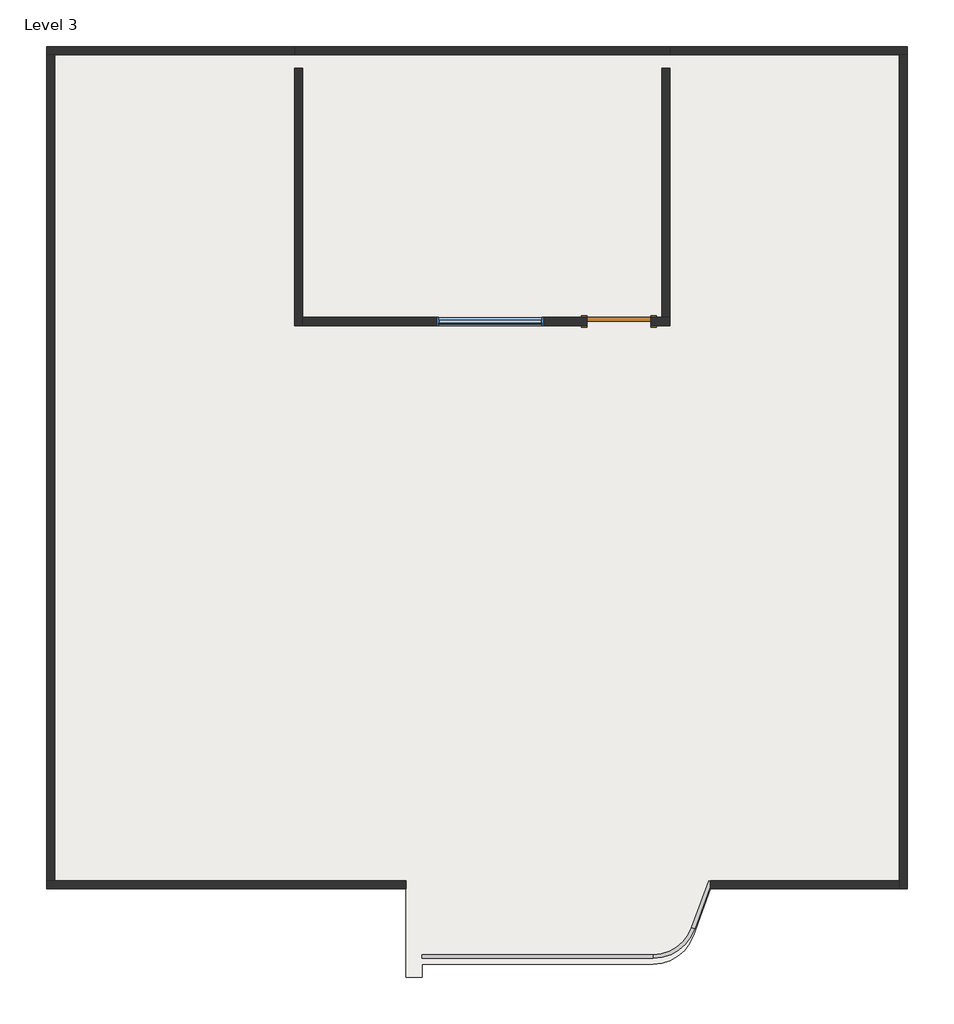
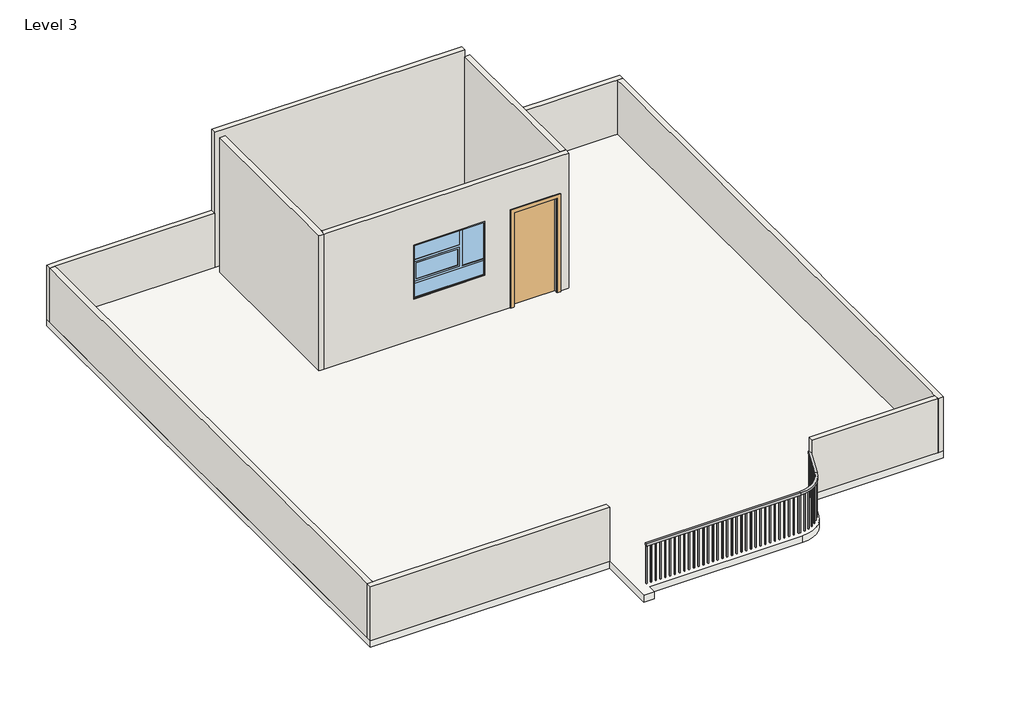
# One storey: 10 walls, 1 door, 1 railing, 1 slab, 1 window.
"""IFC4 building model written with IfcOpenShell, lengths in millimetres."""

from ifc_helpers import new_model, si_unit, point, frame, frame_2d, origin, place, context, project, spatial, polyline, circle_curve, trimmed, segment, composite_curve, outline, extrude, faceted_brep, transform, mapped, element, save
from ifc_brep_helpers import plane_surface, cylinder_surface, revolved_surface, advanced_brep
from components import door_e5f9f3c4, window_awning_variable_5_x4_55050b8f

model = new_model("IFC4")

# Units and contexts
model_context = context("Model", 3, world=origin())
ifc_project = project(units=[si_unit("LENGTHUNIT", "METRE", prefix="MILLI")], contexts=[model_context])

# Site, building, storey
site = spatial("IfcSite", under=ifc_project)
building = spatial("IfcBuilding", under=site)
storey = spatial("IfcBuildingStorey", under=building, Name="Level 3", Elevation=6400.8)

# Door
placement = place(None, origin())
door_shape = door_e5f9f3c4(model_context)
element("IfcDoor", 1, ObjectType="Single-Flush : 36\" x 84\"", at=placement, inside=storey, context=model_context, shape_type="MappedRepresentation", body=[
    mapped(door_shape, transform((-6761.6178125, 9626.366018, 6400.8), x_axis=(1.0, 0.0, 0.0), y_axis=(0.0, 1.0, 0.0), z_axis=(0.0, 0.0, 1.0))),
])

# Railing
element("IfcRailing", 2, ObjectType="Handrail - Rectangular", at=placement, inside=storey, context=model_context, shape_type="SolidModel", body=[
    advanced_brep(
    [(-9561.9678125, 634.766018, 7315.2), (-9561.9678125, 634.766018, 7264.4), (-9561.9678125, 583.966018, 7264.4), (-9561.9678125, 583.966018, 7315.2), (-6278.443289, 634.766018, 7315.2), (-6278.443289, 634.766018, 7264.4), (-6278.443289, 583.966018, 7264.4), (-6278.443289, 583.966018, 7315.2), (-5729.4748599, 1019.1578503, 7264.4), (-5729.4748599, 1019.1578503, 7315.2), (-5681.7384748, 1001.783227, 7264.4), (-5681.7384748, 1001.783227, 7315.2), (-5487.1815204, 1684.8533296, 7315.2), (-5439.4451352, 1667.4787064, 7315.2), (-5439.4451352, 1667.4787064, 7264.4), (-5487.1815204, 1684.8533296, 7264.4)],
    [
        (0, 1),
        (1, 2),
        (2, 3),
        (3, 0),
        (0, 4),
        (4, 5),
        (5, 1),
        (5, 6),
        (6, 2),
        (6, 7),
        (7, 3),
        (7, 4),
        (8, 5, circle_curve(frame((-6278.443289, 1218.966018, 7264.4), z_axis=(0.0, 0.0, -1.0), x_axis=(0.0, -1.0, 0.0)), 584.2)),
        (4, 9, circle_curve(frame((-6278.443289, 1218.966018, 7315.2), z_axis=(0.0, 0.0, 1.0), x_axis=(0.0, -1.0, 0.0)), 584.2)),
        (9, 8),
        (10, 6, circle_curve(frame((-6278.443289, 1218.966018, 7264.4), z_axis=(0.0, 0.0, -1.0), x_axis=(0.0, -1.0, 0.0)), 635.0)),
        (8, 10),
        (11, 7, circle_curve(frame((-6278.443289, 1218.966018, 7315.2), z_axis=(0.0, 0.0, -1.0), x_axis=(0.0, -1.0, 0.0)), 635.0)),
        (10, 11),
        (11, 9),
        (12, 13),
        (13, 14),
        (14, 15),
        (15, 12),
        (9, 12),
        (15, 8),
        (14, 10),
        (13, 11),
    ],
    [
        plane_surface(frame((-9561.9678125, 609.366018, 7315.2), z_axis=(-1.0, 0.0, 0.0), x_axis=(0.0, 1.0, 0.0))),
        plane_surface(frame((-9561.9678125, 634.766018, 7315.2), z_axis=(0.0, 1.0, 0.0), x_axis=(1.0, 0.0, 0.0))),
        plane_surface(frame((-9561.9678125, 634.766018, 7264.4), z_axis=(0.0, 0.0, -1.0), x_axis=(1.0, 0.0, 0.0))),
        plane_surface(frame((-9561.9678125, 583.966018, 7264.4), z_axis=(0.0, -1.0, 0.0), x_axis=(1.0, 0.0, 0.0))),
        plane_surface(frame((-9561.9678125, 583.966018, 7315.2), z_axis=(0.0, 0.0, 1.0), x_axis=(1.0, 0.0, 0.0))),
        revolved_surface(polyline([(-6278.443289, 634.766018, 7315.2), (-6278.443289, 634.766018, 7264.4)]), (-6278.443289, 1218.966018, 7315.2), (0.0, 0.0, 1.0)),
        plane_surface(frame((-6278.443289, 1218.966018, 7264.4), z_axis=(0.0, 0.0, -1.0), x_axis=(0.0, -1.0, 0.0))),
        cylinder_surface(frame((-6278.443289, 1218.966018, 7315.2), z_axis=(0.0, 0.0, 1.0), x_axis=(0.0, -1.0, 0.0)), 635.0),
        plane_surface(frame((-6278.443289, 1218.966018, 7315.2), z_axis=(0.0, 0.0, 1.0), x_axis=(0.0, -1.0, 0.0))),
        plane_surface(frame((-5463.3133278, 1676.166018, 7315.2), z_axis=(0.3420201433256705, 0.9396926207859078, 0.0), x_axis=(0.9396926207859078, -0.3420201433256705, 0.0))),
        plane_surface(frame((-5729.4748599, 1019.1578503, 7315.2), z_axis=(-0.9396926207859079, 0.3420201433256703, 0.0), x_axis=(0.3420201433256703, 0.9396926207859079, 0.0))),
        plane_surface(frame((-5729.4748599, 1019.1578503, 7264.4), z_axis=(0.0, 0.0, -1.0), x_axis=(0.3420201433256703, 0.9396926207859079, 0.0))),
        plane_surface(frame((-5681.7384748, 1001.783227, 7264.4), z_axis=(0.9396926207859079, -0.34202014332567027, 0.0), x_axis=(0.34202014332567027, 0.9396926207859079, 0.0))),
        plane_surface(frame((-5681.7384748, 1001.783227, 7315.2), z_axis=(0.0, 0.0, 1.0), x_axis=(0.34202014332567027, 0.9396926207859079, 0.0))),
    ],
    [
        (0, [[1, 2, 3, 4]]),
        (1, [[-1, 5, 6, 7]]),
        (2, [[-2, -7, 8, 9]]),
        (3, [[-3, -9, 10, 11]]),
        (4, [[-4, -11, 12, -5]]),
        (5, [[13, -6, 14, 15]]),
        (6, [[16, -8, -13, 17]]),
        (7, [[18, -10, -16, 19]]),
        (8, [[-14, -12, -18, 20]]),
        (9, [[21, 22, 23, 24]]),
        (10, [[-15, 25, -24, 26]]),
        (11, [[-17, -26, -23, 27]]),
        (12, [[-19, -27, -22, 28]]),
        (13, [[-20, -28, -21, -25]]),
    ],
),
    extrude(outline(polyline([(-5491.4183577, 1571.0988462), (-5509.3195021, 1577.6143299), (-5502.8040184, 1595.5154743), (-5484.9028739, 1588.9999906), (-5491.4183577, 1571.0988462)])), frame((0.0, 0.0, 6400.8), z_axis=(0.0, 0.0, 1.0), x_axis=(1.0, 0.0, 0.0)), (0.0, 0.0, 1.0), 863.6),
    extrude(outline(polyline([(-5526.1676042, 1475.6260759), (-5544.0687486, 1482.1415596), (-5537.5532649, 1500.0427041), (-5519.6521205, 1493.5272203), (-5526.1676042, 1475.6260759)])), frame((0.0, 0.0, 6400.8), z_axis=(0.0, 0.0, 1.0), x_axis=(1.0, 0.0, 0.0)), (0.0, 0.0, 1.0), 863.6),
    extrude(outline(polyline([(-5560.9168508, 1380.1533056), (-5578.8179952, 1386.6687894), (-5572.3025115, 1404.5699338), (-5554.4013671, 1398.0544501), (-5560.9168508, 1380.1533056)])), frame((0.0, 0.0, 6400.8), z_axis=(0.0, 0.0, 1.0), x_axis=(1.0, 0.0, 0.0)), (0.0, 0.0, 1.0), 863.6),
    extrude(outline(polyline([(-5595.6660973, 1284.6805354), (-5613.5672418, 1291.1960191), (-5607.051758, 1309.0971635), (-5589.1506136, 1302.5816798), (-5595.6660973, 1284.6805354)])), frame((0.0, 0.0, 6400.8), z_axis=(0.0, 0.0, 1.0), x_axis=(1.0, 0.0, 0.0)), (0.0, 0.0, 1.0), 863.6),
    extrude(outline(polyline([(-5630.4153439, 1189.2077651), (-5648.3164883, 1195.7232488), (-5641.8010046, 1213.6243932), (-5623.8998602, 1207.1089095), (-5630.4153439, 1189.2077651)])), frame((0.0, 0.0, 6400.8), z_axis=(0.0, 0.0, 1.0), x_axis=(1.0, 0.0, 0.0)), (0.0, 0.0, 1.0), 863.6),
    extrude(outline(polyline([(-5665.1645905, 1093.7349948), (-5683.0657349, 1100.2504785), (-5676.5502512, 1118.151623), (-5658.6491067, 1111.6361392), (-5665.1645905, 1093.7349948)])), frame((0.0, 0.0, 6400.8), z_axis=(0.0, 0.0, 1.0), x_axis=(1.0, 0.0, 0.0)), (0.0, 0.0, 1.0), 863.6),
    extrude(outline(polyline([(-5712.9373242, 966.7567894), (-5730.452751, 974.2476053), (-5722.9619352, 991.7630322), (-5705.4465083, 984.2722163), (-5712.9373242, 966.7567894)])), frame((0.0, 0.0, 6400.8), z_axis=(0.0, 0.0, 1.0), x_axis=(1.0, 0.0, 0.0)), (0.0, 0.0, 1.0), 863.6),
    extrude(outline(polyline([(-5762.613945, 876.4363417), (-5778.6439673, 886.7291007), (-5768.3512083, 902.7591229), (-5752.3211861, 892.466364), (-5762.613945, 876.4363417)])), frame((0.0, 0.0, 6400.8), z_axis=(0.0, 0.0, 1.0), x_axis=(1.0, 0.0, 0.0)), (0.0, 0.0, 1.0), 863.6),
    extrude(outline(polyline([(-5826.5860214, 795.6086028), (-5840.6863905, 808.4180561), (-5827.8769372, 822.5184252), (-5813.7765681, 809.7089719), (-5826.5860214, 795.6086028)])), frame((0.0, 0.0, 6400.8), z_axis=(0.0, 0.0, 1.0), x_axis=(1.0, 0.0, 0.0)), (0.0, 0.0, 1.0), 863.6),
    extrude(outline(polyline([(-5903.0806608, 726.5135953), (-5914.8606056, 741.4847476), (-5899.8894533, 753.2646924), (-5888.1095085, 738.29354), (-5903.0806608, 726.5135953)])), frame((0.0, 0.0, 6400.8), z_axis=(0.0, 0.0, 1.0), x_axis=(1.0, 0.0, 0.0)), (0.0, 0.0, 1.0), 863.6),
    extrude(outline(polyline([(-5989.9779263, 671.0661861), (-5999.1109828, 687.7841339), (-5982.393035, 696.9171904), (-5973.2599785, 680.1992426), (-5989.9779263, 671.0661861)])), frame((0.0, 0.0, 6400.8), z_axis=(0.0, 0.0, 1.0), x_axis=(1.0, 0.0, 0.0)), (0.0, 0.0, 1.0), 863.6),
    extrude(outline(polyline([(-6084.8695873, 630.8030191), (-6091.1026462, 648.8044489), (-6073.1012164, 655.0375079), (-6066.8681574, 637.0360781), (-6084.8695873, 630.8030191)])), frame((0.0, 0.0, 6400.8), z_axis=(0.0, 0.0, 1.0), x_axis=(1.0, 0.0, 0.0)), (0.0, 0.0, 1.0), 863.6),
    extrude(outline(polyline([(-6185.1258601, 606.8399291), (-6188.2861815, 625.6259576), (-6169.5001529, 628.786279), (-6166.3398316, 610.0002504), (-6185.1258601, 606.8399291)])), frame((0.0, 0.0, 6400.8), z_axis=(0.0, 0.0, 1.0), x_axis=(1.0, 0.0, 0.0)), (0.0, 0.0, 1.0), 863.6),
    extrude(outline(polyline([(-6320.2928125, 599.841018), (-6320.2928125, 618.891018), (-6301.2428125, 618.891018), (-6301.2428125, 599.841018), (-6320.2928125, 599.841018)])), frame((0.0, 0.0, 6400.8), z_axis=(0.0, 0.0, 1.0), x_axis=(1.0, 0.0, 0.0)), (0.0, 0.0, 1.0), 863.6),
    extrude(outline(polyline([(-6421.8928125, 599.841018), (-6421.8928125, 618.891018), (-6402.8428125, 618.891018), (-6402.8428125, 599.841018), (-6421.8928125, 599.841018)])), frame((0.0, 0.0, 6400.8), z_axis=(0.0, 0.0, 1.0), x_axis=(1.0, 0.0, 0.0)), (0.0, 0.0, 1.0), 863.6),
    extrude(outline(polyline([(-6523.4928125, 599.841018), (-6523.4928125, 618.891018), (-6504.4428125, 618.891018), (-6504.4428125, 599.841018), (-6523.4928125, 599.841018)])), frame((0.0, 0.0, 6400.8), z_axis=(0.0, 0.0, 1.0), x_axis=(1.0, 0.0, 0.0)), (0.0, 0.0, 1.0), 863.6),
    extrude(outline(polyline([(-6625.0928125, 599.841018), (-6625.0928125, 618.891018), (-6606.0428125, 618.891018), (-6606.0428125, 599.841018), (-6625.0928125, 599.841018)])), frame((0.0, 0.0, 6400.8), z_axis=(0.0, 0.0, 1.0), x_axis=(1.0, 0.0, 0.0)), (0.0, 0.0, 1.0), 863.6),
    extrude(outline(polyline([(-6726.6928125, 599.841018), (-6726.6928125, 618.891018), (-6707.6428125, 618.891018), (-6707.6428125, 599.841018), (-6726.6928125, 599.841018)])), frame((0.0, 0.0, 6400.8), z_axis=(0.0, 0.0, 1.0), x_axis=(1.0, 0.0, 0.0)), (0.0, 0.0, 1.0), 863.6),
    extrude(outline(polyline([(-6828.2928125, 599.841018), (-6828.2928125, 618.891018), (-6809.2428125, 618.891018), (-6809.2428125, 599.841018), (-6828.2928125, 599.841018)])), frame((0.0, 0.0, 6400.8), z_axis=(0.0, 0.0, 1.0), x_axis=(1.0, 0.0, 0.0)), (0.0, 0.0, 1.0), 863.6),
    extrude(outline(polyline([(-6929.8928125, 599.841018), (-6929.8928125, 618.891018), (-6910.8428125, 618.891018), (-6910.8428125, 599.841018), (-6929.8928125, 599.841018)])), frame((0.0, 0.0, 6400.8), z_axis=(0.0, 0.0, 1.0), x_axis=(1.0, 0.0, 0.0)), (0.0, 0.0, 1.0), 863.6),
    extrude(outline(polyline([(-7031.4928125, 599.841018), (-7031.4928125, 618.891018), (-7012.4428125, 618.891018), (-7012.4428125, 599.841018), (-7031.4928125, 599.841018)])), frame((0.0, 0.0, 6400.8), z_axis=(0.0, 0.0, 1.0), x_axis=(1.0, 0.0, 0.0)), (0.0, 0.0, 1.0), 863.6),
    extrude(outline(polyline([(-7133.0928125, 599.841018), (-7133.0928125, 618.891018), (-7114.0428125, 618.891018), (-7114.0428125, 599.841018), (-7133.0928125, 599.841018)])), frame((0.0, 0.0, 6400.8), z_axis=(0.0, 0.0, 1.0), x_axis=(1.0, 0.0, 0.0)), (0.0, 0.0, 1.0), 863.6),
    extrude(outline(polyline([(-7234.6928125, 599.841018), (-7234.6928125, 618.891018), (-7215.6428125, 618.891018), (-7215.6428125, 599.841018), (-7234.6928125, 599.841018)])), frame((0.0, 0.0, 6400.8), z_axis=(0.0, 0.0, 1.0), x_axis=(1.0, 0.0, 0.0)), (0.0, 0.0, 1.0), 863.6),
    extrude(outline(polyline([(-7336.2928125, 599.841018), (-7336.2928125, 618.891018), (-7317.2428125, 618.891018), (-7317.2428125, 599.841018), (-7336.2928125, 599.841018)])), frame((0.0, 0.0, 6400.8), z_axis=(0.0, 0.0, 1.0), x_axis=(1.0, 0.0, 0.0)), (0.0, 0.0, 1.0), 863.6),
    extrude(outline(polyline([(-7437.8928125, 599.841018), (-7437.8928125, 618.891018), (-7418.8428125, 618.891018), (-7418.8428125, 599.841018), (-7437.8928125, 599.841018)])), frame((0.0, 0.0, 6400.8), z_axis=(0.0, 0.0, 1.0), x_axis=(1.0, 0.0, 0.0)), (0.0, 0.0, 1.0), 863.6),
    extrude(outline(polyline([(-7539.4928125, 599.841018), (-7539.4928125, 618.891018), (-7520.4428125, 618.891018), (-7520.4428125, 599.841018), (-7539.4928125, 599.841018)])), frame((0.0, 0.0, 6400.8), z_axis=(0.0, 0.0, 1.0), x_axis=(1.0, 0.0, 0.0)), (0.0, 0.0, 1.0), 863.6),
    extrude(outline(polyline([(-7641.0928125, 599.841018), (-7641.0928125, 618.891018), (-7622.0428125, 618.891018), (-7622.0428125, 599.841018), (-7641.0928125, 599.841018)])), frame((0.0, 0.0, 6400.8), z_axis=(0.0, 0.0, 1.0), x_axis=(1.0, 0.0, 0.0)), (0.0, 0.0, 1.0), 863.6),
    extrude(outline(polyline([(-7742.6928125, 599.841018), (-7742.6928125, 618.891018), (-7723.6428125, 618.891018), (-7723.6428125, 599.841018), (-7742.6928125, 599.841018)])), frame((0.0, 0.0, 6400.8), z_axis=(0.0, 0.0, 1.0), x_axis=(1.0, 0.0, 0.0)), (0.0, 0.0, 1.0), 863.6),
    extrude(outline(polyline([(-7844.2928125, 599.841018), (-7844.2928125, 618.891018), (-7825.2428125, 618.891018), (-7825.2428125, 599.841018), (-7844.2928125, 599.841018)])), frame((0.0, 0.0, 6400.8), z_axis=(0.0, 0.0, 1.0), x_axis=(1.0, 0.0, 0.0)), (0.0, 0.0, 1.0), 863.6),
    extrude(outline(polyline([(-7945.8928125, 599.841018), (-7945.8928125, 618.891018), (-7926.8428125, 618.891018), (-7926.8428125, 599.841018), (-7945.8928125, 599.841018)])), frame((0.0, 0.0, 6400.8), z_axis=(0.0, 0.0, 1.0), x_axis=(1.0, 0.0, 0.0)), (0.0, 0.0, 1.0), 863.6),
    extrude(outline(polyline([(-8047.4928125, 599.841018), (-8047.4928125, 618.891018), (-8028.4428125, 618.891018), (-8028.4428125, 599.841018), (-8047.4928125, 599.841018)])), frame((0.0, 0.0, 6400.8), z_axis=(0.0, 0.0, 1.0), x_axis=(1.0, 0.0, 0.0)), (0.0, 0.0, 1.0), 863.6),
    extrude(outline(polyline([(-8149.0928125, 599.841018), (-8149.0928125, 618.891018), (-8130.0428125, 618.891018), (-8130.0428125, 599.841018), (-8149.0928125, 599.841018)])), frame((0.0, 0.0, 6400.8), z_axis=(0.0, 0.0, 1.0), x_axis=(1.0, 0.0, 0.0)), (0.0, 0.0, 1.0), 863.6),
    extrude(outline(polyline([(-8250.6928125, 599.841018), (-8250.6928125, 618.891018), (-8231.6428125, 618.891018), (-8231.6428125, 599.841018), (-8250.6928125, 599.841018)])), frame((0.0, 0.0, 6400.8), z_axis=(0.0, 0.0, 1.0), x_axis=(1.0, 0.0, 0.0)), (0.0, 0.0, 1.0), 863.6),
    extrude(outline(polyline([(-8352.2928125, 599.841018), (-8352.2928125, 618.891018), (-8333.2428125, 618.891018), (-8333.2428125, 599.841018), (-8352.2928125, 599.841018)])), frame((0.0, 0.0, 6400.8), z_axis=(0.0, 0.0, 1.0), x_axis=(1.0, 0.0, 0.0)), (0.0, 0.0, 1.0), 863.6),
    extrude(outline(polyline([(-8453.8928125, 599.841018), (-8453.8928125, 618.891018), (-8434.8428125, 618.891018), (-8434.8428125, 599.841018), (-8453.8928125, 599.841018)])), frame((0.0, 0.0, 6400.8), z_axis=(0.0, 0.0, 1.0), x_axis=(1.0, 0.0, 0.0)), (0.0, 0.0, 1.0), 863.6),
    extrude(outline(polyline([(-8555.4928125, 599.841018), (-8555.4928125, 618.891018), (-8536.4428125, 618.891018), (-8536.4428125, 599.841018), (-8555.4928125, 599.841018)])), frame((0.0, 0.0, 6400.8), z_axis=(0.0, 0.0, 1.0), x_axis=(1.0, 0.0, 0.0)), (0.0, 0.0, 1.0), 863.6),
    extrude(outline(polyline([(-8657.0928125, 599.841018), (-8657.0928125, 618.891018), (-8638.0428125, 618.891018), (-8638.0428125, 599.841018), (-8657.0928125, 599.841018)])), frame((0.0, 0.0, 6400.8), z_axis=(0.0, 0.0, 1.0), x_axis=(1.0, 0.0, 0.0)), (0.0, 0.0, 1.0), 863.6),
    extrude(outline(polyline([(-8758.6928125, 599.841018), (-8758.6928125, 618.891018), (-8739.6428125, 618.891018), (-8739.6428125, 599.841018), (-8758.6928125, 599.841018)])), frame((0.0, 0.0, 6400.8), z_axis=(0.0, 0.0, 1.0), x_axis=(1.0, 0.0, 0.0)), (0.0, 0.0, 1.0), 863.6),
    extrude(outline(polyline([(-8860.2928125, 599.841018), (-8860.2928125, 618.891018), (-8841.2428125, 618.891018), (-8841.2428125, 599.841018), (-8860.2928125, 599.841018)])), frame((0.0, 0.0, 6400.8), z_axis=(0.0, 0.0, 1.0), x_axis=(1.0, 0.0, 0.0)), (0.0, 0.0, 1.0), 863.6),
    extrude(outline(polyline([(-8961.8928125, 599.841018), (-8961.8928125, 618.891018), (-8942.8428125, 618.891018), (-8942.8428125, 599.841018), (-8961.8928125, 599.841018)])), frame((0.0, 0.0, 6400.8), z_axis=(0.0, 0.0, 1.0), x_axis=(1.0, 0.0, 0.0)), (0.0, 0.0, 1.0), 863.6),
    extrude(outline(polyline([(-9063.4928125, 599.841018), (-9063.4928125, 618.891018), (-9044.4428125, 618.891018), (-9044.4428125, 599.841018), (-9063.4928125, 599.841018)])), frame((0.0, 0.0, 6400.8), z_axis=(0.0, 0.0, 1.0), x_axis=(1.0, 0.0, 0.0)), (0.0, 0.0, 1.0), 863.6),
    extrude(outline(polyline([(-9165.0928125, 599.841018), (-9165.0928125, 618.891018), (-9146.0428125, 618.891018), (-9146.0428125, 599.841018), (-9165.0928125, 599.841018)])), frame((0.0, 0.0, 6400.8), z_axis=(0.0, 0.0, 1.0), x_axis=(1.0, 0.0, 0.0)), (0.0, 0.0, 1.0), 863.6),
    extrude(outline(polyline([(-9266.6928125, 599.841018), (-9266.6928125, 618.891018), (-9247.6428125, 618.891018), (-9247.6428125, 599.841018), (-9266.6928125, 599.841018)])), frame((0.0, 0.0, 6400.8), z_axis=(0.0, 0.0, 1.0), x_axis=(1.0, 0.0, 0.0)), (0.0, 0.0, 1.0), 863.6),
    extrude(outline(polyline([(-9368.2928125, 599.841018), (-9368.2928125, 618.891018), (-9349.2428125, 618.891018), (-9349.2428125, 599.841018), (-9368.2928125, 599.841018)])), frame((0.0, 0.0, 6400.8), z_axis=(0.0, 0.0, 1.0), x_axis=(1.0, 0.0, 0.0)), (0.0, 0.0, 1.0), 863.6),
    extrude(outline(polyline([(-9469.8928125, 599.841018), (-9469.8928125, 618.891018), (-9450.8428125, 618.891018), (-9450.8428125, 599.841018), (-9469.8928125, 599.841018)])), frame((0.0, 0.0, 6400.8), z_axis=(0.0, 0.0, 1.0), x_axis=(1.0, 0.0, 0.0)), (0.0, 0.0, 1.0), 863.6),
    extrude(outline(polyline([(-5699.913837, 998.2622245), (-5717.8149815, 1004.7777083), (-5711.2994977, 1022.6788527), (-5693.3983533, 1016.163369), (-5699.913837, 998.2622245)])), frame((0.0, 0.0, 6400.8), z_axis=(0.0, 0.0, 1.0), x_axis=(1.0, 0.0, 0.0)), (0.0, 0.0, 1.0), 863.6),
    extrude(outline(polyline([(-6287.968289, 599.841018), (-6287.968289, 618.891018), (-6268.918289, 618.891018), (-6268.918289, 599.841018), (-6287.968289, 599.841018)])), frame((0.0, 0.0, 6400.8), z_axis=(0.0, 0.0, 1.0), x_axis=(1.0, 0.0, 0.0)), (0.0, 0.0, 1.0), 863.6),
    extrude(outline(polyline([(-5460.8782393, 1655.0071317), (-5478.7793837, 1661.5226154), (-5472.2639, 1679.4237599), (-5454.3627556, 1672.9082761), (-5460.8782393, 1655.0071317)])), frame((0.0, 0.0, 6400.8), z_axis=(0.0, 0.0, 1.0), x_axis=(1.0, 0.0, 0.0)), (0.0, 0.0, 1.0), 863.6),
    extrude(outline(polyline([(-9561.9678125, 599.841018), (-9561.9678125, 618.891018), (-9542.9178125, 618.891018), (-9542.9178125, 599.841018), (-9561.9678125, 599.841018)])), frame((0.0, 0.0, 6400.8), z_axis=(0.0, 0.0, 1.0), x_axis=(1.0, 0.0, 0.0)), (0.0, 0.0, 1.0), 863.6),
])

# Slab
element("IfcSlab", 3, ObjectType="6\" floor", at=placement, inside=storey, context=model_context, shape_type="SweptSolid", body=[
    extrude(outline(composite_curve([segment(polyline([(-2665.8678125, 13531.616018), (-2665.8678125, 1568.216018), (-5463.3133278, 1568.216018), (-5705.6066674, 902.5205386)]), True, "CONTINUOUS"), segment(trimmed(circle_curve(frame_2d((-6278.443289, 1111.016018)), 609.6), [point((-5705.6066674, 902.5205386))], [point((-6278.443289, 501.416018))], False, "CARTESIAN"), True, "CONTINUOUS"), segment(polyline([(-6278.443289, 501.416018), (-9561.9678125, 501.416018), (-9561.9678125, 310.916018), (-9790.5678125, 310.916018), (-9790.5678125, 1568.216018), (-14895.9678125, 1568.216018), (-14895.9678125, 13531.616018), (-2665.8678125, 13531.616018)]), True, "CONTINUOUS")], self_intersect=False)), frame((0.0, 0.0, 6248.4), z_axis=(0.0, 0.0, 1.0), x_axis=(1.0, 0.0, 0.0)), (0.0, 0.0, 1.0), 152.4),
])

# Walls
element("IfcWall", 4, ObjectType="4.5\" wall", at=placement, inside=storey, context=model_context, shape_type="Brep", body=[
    faceted_brep([(-2665.8678125, 13531.616018, 6400.8), (-6037.7178125, 13531.616018, 6400.8), (-6037.7178125, 13531.616018, 7620.0), (-2894.4678125, 13531.616018, 7620.0), (-2665.8678125, 13531.616018, 7620.0), (-2665.8678125, 13417.316018, 6400.8), (-2665.8678125, 13417.316018, 7620.0), (-2780.1678125, 13417.316018, 7620.0), (-2894.4678125, 13417.316018, 7620.0), (-6037.7178125, 13417.316018, 7620.0), (-6037.7178125, 13417.316018, 6400.8), (-2894.4678125, 13417.316018, 6400.8), (-2780.1678125, 13417.316018, 6400.8)], [[[0, 1, 2, 3, 4]], [[5, 6, 7, 8, 9, 10, 11, 12]], [[1, 0, 5, 12, 11, 10]], [[2, 1, 10, 9]], [[4, 3, 2, 9, 8, 7, 6]], [[0, 4, 6, 5]]]),
])
element("IfcWall", 5, ObjectType="4.5\" wall", at=placement, inside=storey, context=model_context, shape_type="Brep", body=[
    faceted_brep([(-2665.8678125, 1568.216018, 6400.8), (-2665.8678125, 1873.016018, 6400.8), (-2665.8678125, 5930.666018, 6400.8), (-2665.8678125, 6235.466018, 6400.8), (-2665.8678125, 9397.766018, 6400.8), (-2665.8678125, 9702.566018, 6400.8), (-2665.8678125, 13226.816018, 6400.8), (-2665.8678125, 13303.016018, 6400.8), (-2665.8678125, 13417.316018, 6400.8), (-2665.8678125, 13417.316018, 7620.0), (-2665.8678125, 13226.816018, 7620.0), (-2665.8678125, 9702.566018, 7620.0), (-2665.8678125, 9397.766018, 7620.0), (-2665.8678125, 6235.466018, 7620.0), (-2665.8678125, 5930.666018, 7620.0), (-2665.8678125, 1873.016018, 7620.0), (-2665.8678125, 1568.216018, 7620.0), (-2780.1678125, 1568.216018, 6400.8), (-2780.1678125, 1568.216018, 7620.0), (-2780.1678125, 1682.516018, 7620.0), (-2780.1678125, 1873.016018, 7620.0), (-2780.1678125, 5930.666018, 7620.0), (-2780.1678125, 6235.466018, 7620.0), (-2780.1678125, 9397.766018, 7620.0), (-2780.1678125, 9702.566018, 7620.0), (-2780.1678125, 13226.816018, 7620.0), (-2780.1678125, 13417.316018, 7620.0), (-2780.1678125, 13417.316018, 6400.8), (-2780.1678125, 13303.016018, 6400.8), (-2780.1678125, 13226.816018, 6400.8), (-2780.1678125, 9702.566018, 6400.8), (-2780.1678125, 9397.766018, 6400.8), (-2780.1678125, 6235.466018, 6400.8), (-2780.1678125, 5930.666018, 6400.8), (-2780.1678125, 1873.016018, 6400.8), (-2780.1678125, 1682.516018, 6400.8)], [[[0, 1, 2, 3, 4, 5, 6, 7, 8, 9, 10, 11, 12, 13, 14, 15, 16]], [[17, 18, 19, 20, 21, 22, 23, 24, 25, 26, 27, 28, 29, 30, 31, 32, 33, 34, 35]], [[8, 7, 6, 5, 4, 3, 2, 1, 0, 17, 35, 34, 33, 32, 31, 30, 29, 28, 27]], [[16, 15, 14, 13, 12, 11, 10, 9, 26, 25, 24, 23, 22, 21, 20, 19, 18]], [[9, 8, 27, 26]], [[0, 16, 18, 17]]]),
])
element("IfcWall", 6, ObjectType="4.5\" wall", at=placement, inside=storey, context=model_context, shape_type="Brep", body=[
    faceted_brep([(-5463.3133278, 1568.216018, 6400.8), (-2894.4678125, 1568.216018, 6400.8), (-2780.1678125, 1568.216018, 6400.8), (-2780.1678125, 1568.216018, 7620.0), (-2894.4678125, 1568.216018, 7620.0), (-5463.3133278, 1568.216018, 7620.0), (-5463.3133278, 1682.516018, 6400.8), (-5463.3133278, 1682.516018, 7620.0), (-2894.4678125, 1682.516018, 7620.0), (-2780.1678125, 1682.516018, 7620.0), (-2780.1678125, 1682.516018, 6400.8), (-2894.4678125, 1682.516018, 6400.8)], [[[0, 1, 2, 3, 4, 5]], [[6, 7, 8, 9, 10, 11]], [[2, 1, 0, 6, 11, 10]], [[5, 4, 3, 9, 8, 7]], [[0, 5, 7, 6]], [[3, 2, 10, 9]]]),
])
element("IfcWall", 7, ObjectType="4.5\" wall", at=placement, inside=storey, context=model_context, shape_type="Brep", body=[
    faceted_brep([(-14895.9678125, 1568.216018, 6400.8), (-14667.3678125, 1568.216018, 6400.8), (-9790.5678125, 1568.216018, 6400.8), (-9790.5678125, 1568.216018, 7218.0977729), (-9790.5678125, 1568.216018, 7620.0), (-14629.2678125, 1568.216018, 7620.0), (-14895.9678125, 1568.216018, 7620.0), (-14895.9678125, 1682.516018, 6400.8), (-14895.9678125, 1682.516018, 7620.0), (-14781.6678125, 1682.516018, 7620.0), (-14629.2678125, 1682.516018, 7620.0), (-9790.5678125, 1682.516018, 7620.0), (-9790.5678125, 1682.516018, 7218.0977729), (-9790.5678125, 1682.516018, 6400.8), (-14629.2678125, 1682.516018, 6400.8), (-14667.3678125, 1682.516018, 6400.8), (-14781.6678125, 1682.516018, 6400.8)], [[[0, 1, 2, 3, 4, 5, 6]], [[7, 8, 9, 10, 11, 12, 13, 14, 15, 16]], [[2, 1, 0, 7, 16, 15, 14, 13]], [[6, 5, 4, 11, 10, 9, 8]], [[0, 6, 8, 7]], [[4, 3, 2, 13, 12, 11]]]),
])
element("IfcWall", 8, ObjectType="4.5\" wall", at=placement, inside=storey, context=model_context, shape_type="Brep", body=[
    faceted_brep([(-14895.9678125, 13417.316018, 6400.8), (-14895.9678125, 9645.416018, 6400.8), (-14895.9678125, 9340.616018, 6400.8), (-14895.9678125, 6235.466018, 6400.8), (-14895.9678125, 5930.666018, 6400.8), (-14895.9678125, 1682.516018, 6400.8), (-14895.9678125, 1682.516018, 7620.0), (-14895.9678125, 1796.816018, 7620.0), (-14895.9678125, 5930.666018, 7620.0), (-14895.9678125, 6235.466018, 7620.0), (-14895.9678125, 9340.616018, 7620.0), (-14895.9678125, 9645.416018, 7620.0), (-14895.9678125, 13303.016018, 7620.0), (-14895.9678125, 13417.316018, 7620.0), (-14781.6678125, 13417.316018, 6400.8), (-14781.6678125, 13417.316018, 7620.0), (-14781.6678125, 13303.016018, 7620.0), (-14781.6678125, 9645.416018, 7620.0), (-14781.6678125, 9340.616018, 7620.0), (-14781.6678125, 6235.466018, 7620.0), (-14781.6678125, 5930.666018, 7620.0), (-14781.6678125, 1796.816018, 7620.0), (-14781.6678125, 1682.516018, 7620.0), (-14781.6678125, 1682.516018, 6400.8), (-14781.6678125, 1796.816018, 6400.8), (-14781.6678125, 5930.666018, 6400.8), (-14781.6678125, 6235.466018, 6400.8), (-14781.6678125, 9340.616018, 6400.8), (-14781.6678125, 9645.416018, 6400.8), (-14781.6678125, 13303.016018, 6400.8)], [[[0, 1, 2, 3, 4, 5, 6, 7, 8, 9, 10, 11, 12, 13]], [[14, 15, 16, 17, 18, 19, 20, 21, 22, 23, 24, 25, 26, 27, 28, 29]], [[5, 4, 3, 2, 1, 0, 14, 29, 28, 27, 26, 25, 24, 23]], [[13, 12, 11, 10, 9, 8, 7, 6, 22, 21, 20, 19, 18, 17, 16, 15]], [[6, 5, 23, 22]], [[0, 13, 15, 14]]]),
])
element("IfcWall", 9, ObjectType="4.5\" wall", at=placement, inside=storey, context=model_context, shape_type="Brep", body=[
    faceted_brep([(-11371.7178125, 13226.816018, 6400.8), (-11371.7178125, 9702.566018, 6400.8), (-11371.7178125, 9645.416018, 6400.8), (-11371.7178125, 9569.216018, 6400.8), (-11371.7178125, 9569.216018, 9448.8), (-11371.7178125, 9702.566018, 9448.8), (-11371.7178125, 13226.816018, 9448.8), (-11257.4178125, 13226.816018, 6400.8), (-11257.4178125, 13226.816018, 9448.8), (-11257.4178125, 9702.566018, 9448.8), (-11257.4178125, 9683.516018, 9448.8), (-11257.4178125, 9569.216018, 9448.8), (-11257.4178125, 9569.216018, 6400.8), (-11257.4178125, 9683.516018, 6400.8), (-11257.4178125, 9702.566018, 6400.8), (-11314.5678125, 13226.816018, 6400.8), (-11314.5678125, 9569.216018, 6400.8)], [[[0, 1, 2, 3, 4, 5, 6]], [[7, 8, 9, 10, 11, 12, 13, 14]], [[3, 2, 1, 0, 15, 7, 14, 13, 12, 16]], [[6, 5, 4, 11, 10, 9, 8]], [[0, 6, 8, 7, 15]], [[4, 3, 16, 12, 11]]]),
])
element("IfcWall", 10, ObjectType="4.5\" wall", at=placement, inside=storey, context=model_context, shape_type="Brep", body=[
    faceted_brep([(-6304.4178125, 9569.216018, 8534.4), (-6304.4178125, 9569.216018, 6400.8), (-6209.1678125, 9569.216018, 6400.8), (-6094.8678125, 9569.216018, 6400.8), (-6037.7178125, 9569.216018, 6400.8), (-6037.7178125, 9569.216018, 9448.8), (-6209.1678125, 9569.216018, 9448.8), (-11200.2678125, 9569.216018, 9448.8), (-11257.4178125, 9569.216018, 9448.8), (-11257.4178125, 9569.216018, 6400.8), (-11200.2678125, 9569.216018, 6400.8), (-7218.8178125, 9569.216018, 6400.8), (-7218.8178125, 9569.216018, 8534.4), (-9352.4178125, 9569.216018, 8534.4), (-7828.4178125, 9569.216018, 8534.4), (-7828.4178125, 9569.216018, 7315.2), (-9352.4178125, 9569.216018, 7315.2), (-6037.7178125, 9683.516018, 6400.8), (-6152.0178125, 9683.516018, 6400.8), (-6209.1678125, 9683.516018, 6400.8), (-6304.4178125, 9683.516018, 6400.8), (-6304.4178125, 9683.516018, 8534.4), (-7218.8178125, 9683.516018, 8534.4), (-7218.8178125, 9683.516018, 6400.8), (-11200.2678125, 9683.516018, 6400.8), (-11257.4178125, 9683.516018, 6400.8), (-11257.4178125, 9683.516018, 9448.8), (-11200.2678125, 9683.516018, 9448.8), (-6209.1678125, 9683.516018, 9448.8), (-6152.0178125, 9683.516018, 9448.8), (-6037.7178125, 9683.516018, 9448.8), (-9352.4178125, 9683.516018, 8534.4), (-9352.4178125, 9683.516018, 7315.2), (-7828.4178125, 9683.516018, 7315.2), (-7828.4178125, 9683.516018, 8534.4), (-6037.7178125, 9645.416018, 6400.8)], [[[0, 1, 2, 3, 4, 5, 6, 7, 8, 9, 10, 11, 12], [13, 14, 15, 16]], [[17, 18, 19, 20, 21, 22, 23, 24, 25, 26, 27, 28, 29, 30], [31, 32, 33, 34]], [[11, 10, 9, 25, 24, 23]], [[4, 3, 2, 1, 20, 19, 18, 17, 35]], [[8, 7, 6, 5, 30, 29, 28, 27, 26]], [[9, 8, 26, 25]], [[5, 4, 35, 17, 30]], [[21, 20, 1, 0]], [[22, 21, 0, 12]], [[23, 22, 12, 11]], [[32, 31, 13, 16]], [[33, 32, 16, 15]], [[34, 33, 15, 14]], [[31, 34, 14, 13]]]),
])
element("IfcWall", 11, ObjectType="4.5\" wall", at=placement, inside=storey, context=model_context, shape_type="Brep", body=[
    faceted_brep([(-6037.7178125, 9683.516018, 6400.8), (-6037.7178125, 9702.566018, 6400.8), (-6037.7178125, 13226.816018, 6400.8), (-6037.7178125, 13226.816018, 9448.8), (-6037.7178125, 9702.566018, 9448.8), (-6037.7178125, 9683.516018, 9448.8), (-6152.0178125, 9683.516018, 6400.8), (-6152.0178125, 9683.516018, 9448.8), (-6152.0178125, 9702.566018, 9448.8), (-6152.0178125, 13226.816018, 9448.8), (-6152.0178125, 13226.816018, 6400.8), (-6152.0178125, 9702.566018, 6400.8), (-6094.8678125, 13226.816018, 6400.8)], [[[0, 1, 2, 3, 4, 5]], [[6, 7, 8, 9, 10, 11]], [[2, 1, 0, 6, 11, 10, 12]], [[3, 2, 12, 10, 9]], [[5, 4, 3, 9, 8, 7]], [[0, 5, 7, 6]]]),
])
element("IfcWall", 12, ObjectType="4.5\" wall", at=placement, inside=storey, context=model_context, shape_type="Brep", body=[
    faceted_brep([(-11371.7178125, 13531.616018, 6400.8), (-14591.1678125, 13531.616018, 6400.8), (-14667.3678125, 13531.616018, 6400.8), (-14895.9678125, 13531.616018, 6400.8), (-14895.9678125, 13531.616018, 7620.0), (-14591.1678125, 13531.616018, 7620.0), (-11371.7178125, 13531.616018, 7620.0), (-11371.7178125, 13417.316018, 6400.8), (-11371.7178125, 13417.316018, 7620.0), (-14591.1678125, 13417.316018, 7620.0), (-14781.6678125, 13417.316018, 7620.0), (-14895.9678125, 13417.316018, 7620.0), (-14895.9678125, 13417.316018, 6400.8), (-14781.6678125, 13417.316018, 6400.8), (-14667.3678125, 13417.316018, 6400.8), (-14591.1678125, 13417.316018, 6400.8)], [[[0, 1, 2, 3, 4, 5, 6]], [[7, 8, 9, 10, 11, 12, 13, 14, 15]], [[3, 2, 1, 0, 7, 15, 14, 13, 12]], [[6, 5, 4, 11, 10, 9, 8]], [[0, 6, 8, 7]], [[4, 3, 12, 11]]]),
])
element("IfcWall", 13, ObjectType="4.5\" wall", at=placement, inside=storey, context=model_context, shape_type="Brep", body=[
    faceted_brep([(-6037.7178125, 13531.616018, 6400.8), (-11371.7178125, 13531.616018, 6400.8), (-11371.7178125, 13531.616018, 7620.0), (-11371.7178125, 13531.616018, 9448.8), (-6037.7178125, 13531.616018, 9448.8), (-6037.7178125, 13531.616018, 7620.0), (-6037.7178125, 13417.316018, 6400.8), (-6037.7178125, 13417.316018, 7620.0), (-6037.7178125, 13417.316018, 9448.8), (-6266.3178125, 13417.316018, 9448.8), (-9504.8178125, 13417.316018, 9448.8), (-9733.4178125, 13417.316018, 9448.8), (-11143.1178125, 13417.316018, 9448.8), (-11371.7178125, 13417.316018, 9448.8), (-11371.7178125, 13417.316018, 7620.0), (-11371.7178125, 13417.316018, 6400.8), (-11143.1178125, 13417.316018, 6400.8), (-9733.4178125, 13417.316018, 6400.8), (-9504.8178125, 13417.316018, 6400.8), (-6266.3178125, 13417.316018, 6400.8)], [[[0, 1, 2, 3, 4, 5]], [[6, 7, 8, 9, 10, 11, 12, 13, 14, 15, 16, 17, 18, 19]], [[1, 0, 6, 19, 18, 17, 16, 15]], [[3, 2, 1, 15, 14, 13]], [[4, 3, 13, 12, 11, 10, 9, 8]], [[0, 5, 4, 8, 7, 6]]]),
])

# Window
window_awning_variable_5_x4_shape = window_awning_variable_5_x4_55050b8f(model_context)
element("IfcWindow", 14, ObjectType="Window-Awning-Variable : 5'x4'", at=placement, inside=storey, context=model_context, shape_type="MappedRepresentation", body=[
    mapped(window_awning_variable_5_x4_shape, transform((-8590.4178125, 9626.366018, 6400.8), x_axis=(-1.0, 0.0, 0.0), y_axis=(0.0, -1.0, 0.0), z_axis=(0.0, 0.0, 1.0))),
])

save(model, "model.ifc")

# Revit data of these elements
# Type "Single-Flush : 36\" x 84\""
#   Type Mark = "1"
#   Construction Type Id = "MDOOR"
#   Assembly Code = "C1020"
#   Analytic Construction = "Metal"
#   Thickness = 0' - 2"
#   Heat Transfer Coefficient (U) = 0.651978 BTU/(h·ft²·°F)
#   Height = 7' - 0"
#   Trim Projection Ext = 0' - 1"
#   Trim Projection Int = 0' - 1"
#   Trim Width = 0' - 3"
#   Width = 3' - 0"
#   Define Thermal Properties by = 1
#   Define Thermal Properties by = 1
#   Door Material = Door - Panel
#   Frame Material = Door - Frame
#   Visual Light Transmittance = 0
#   Solar Heat Gain Coefficient = 0
#   Function = (empty or 0)
#   Wall Closure = (empty or 0)
# Type "Handrail - Rectangular"
#   Assembly Code = "C2010400"
#   built-in parameter 1008612 = 0.0416667 (stored number, unit not read)
#   built-in parameter 1008611 = 0.0416667 (stored number, unit not read)
#   built-in parameter 1008609 = 0.333333 (stored number, unit not read)
#   built-in parameter 1008604 = 0.166667 (stored number, unit not read)
#   built-in parameter 1008603 = 0.166667 (stored number, unit not read)
#   Railing Height = 3' - 0"
#   built-in parameter 1008630 = 2
#   built-in parameter 1008610 = 2
#   built-in parameter 1008618 = Baluster - Square : 3/4"
# Type "6\" floor"
#   Assembly Code = "B1010"
#   Function = 0
#   Layers, outside or top first: 0' - 6" "Gypsum Wall Board" (function 1)
# Type "4.5\" wall"
#   Assembly Code = "B2010"
#   Layers, outside or top first: 0' - 4 1/2" "Gypsum Wall Board" (function 1)
# Type "Window-Awning-Variable : 5'x4'"
#   Type Mark = "23"
#   Fire Rating = "0.5h"
#   Assembly Code = "B2020100"
#   Analytic Construction = "Double glazing - domestic"
#   Window Inset [instance default] = 0' - 0 5/8"
#   Wall Thickness [instance default] = 0' - 6"
#   Visual Light Transmittance = 0.81
#   Transom Height Ratio = 0.3
#   Transom Height = 1' - 2.4"
#   Thermal Resistance (R) = 1.8146 (h·ft²·°F)/BTU
#   Solar Heat Gain Coefficient = 0.76
#   Rough Width = 5' - 0 1/2"
#   Rough Height = 4' - 0 1/2"
#   Opening Window Width = 3' - 4"
#   Opening Window Height = 1' - 7.2"
#   Heat Transfer Coefficient (U) = 0.5511 BTU/(h·ft²·°F)
#   Height = 4' - 0"
#   Frame Gap 3 [instance default] = 0' - 1 83/128"
#   Frame Gap 2 [instance default] = 0' - 0 5/8"
#   Frame Gap 1 = 0' - 1 51/128"
#   Fixed Window Width = 1' - 8"
#   Default Sill Height = 3' - 0"
#   Width = 5' - 0"
#   Frame Material = Metal - Aluminum
#   Glass Panel Material = Glass
#   Wall Closure = (empty or 0)
# Element 1 (IfcDoor, "Single-Flush : 36\" x 84\"")
#   Phase Created = New Construction
#   Materials on its faces: "Door - Frame", "Door - Panel"
# Element 2 (IfcRailing, "Handrail - Rectangular")
#   Phase Created = New Construction
# Element 3 (IfcSlab, "6\" floor")
#   Height Offset From Level = 0' - 0"
#   Phase Created = New Construction
#   Materials on its faces: "Gypsum Wall Board"
# Elements 4, 5, 6, 7, 8, 12 (IfcWall, "4.5\" wall")
#   Top Offset = 0' - 0"
#   Base Offset = 0' - 0"
#   wall height = 4' - 0"
#   Phase Created = New Construction
#   Base Constraint = Level 3
#   Top Constraint = Level 4
#   Materials on its faces: "Gypsum Wall Board"
# Elements 9, 10, 11, 13 (IfcWall, "4.5\" wall")
#   Top Offset = 0' - 0"
#   Base Offset = 0' - 0"
#   wall height = 10' - 0"
#   Phase Created = New Construction
#   Base Constraint = Level 3
#   Top Constraint = Level 5
#   Materials on its faces: "Gypsum Wall Board"
# Element 14 (IfcWindow, "Window-Awning-Variable : 5'x4'")
#   Mark = "21"
#   Window Inset = 0' - 0 5/8"
#   Frame Gap 3 = 0' - 1 83/128"
#   Frame Gap 2 = 0' - 0 5/8"
#   Phase Created = New Construction
#   Materials on its faces: "Glass", "Metal - Aluminum"
# Materials
#   "Door - Panel": class "Wood", colour RGB 210 159 95, transparency 0, Cost = 0
#   "Door - Frame": colour RGB 118 70 51, transparency 0, Cost = 0
#   "Gypsum Wall Board": class "Generic", colour RGB 127 127 127, transparency 0, Description = "Gypsum Wall Board", Cost = 0
#   "Metal - Aluminum": class "Metal", colour RGB 247 247 247, transparency 0
#   "Glass": class "Glass", colour RGB 0 128 192, transparency 0.75, Description = "Soda Lime Glass", Cost = 0
